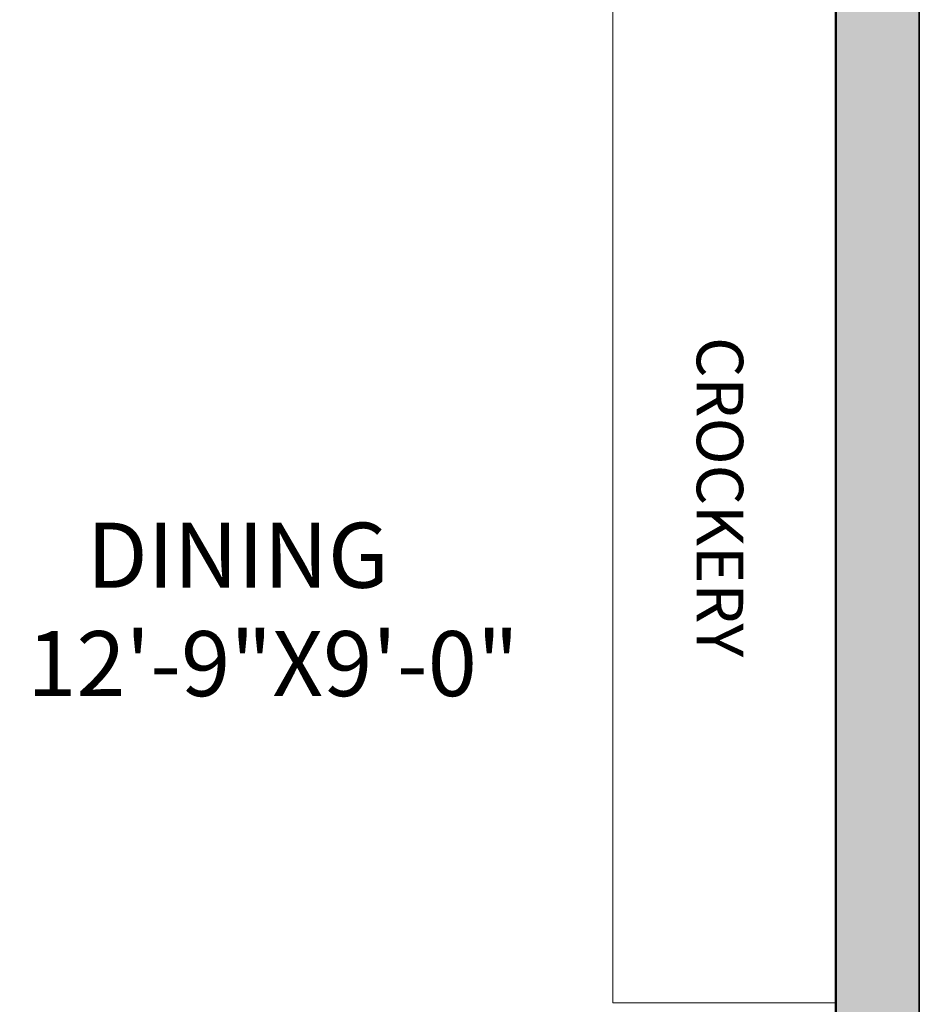
# Model space of a CAD drawing. Units: inches. Extents: x 1734 to 4011, y 1071 to 1891.
# Tile 8 of 27: x 2022 to 2119, y 1650 to 1756. Entities that reach past the tile are written whole.
import ezdxf

# ---------------------------------------------------------------- set-up
doc = ezdxf.new("R2010")
doc.units = ezdxf.units.IN
for name, color, linetype, lineweight in [('A-AREA-IDEN', 3, 'Continuous', 18), ('A-FURN', 8, 'Continuous', 18), ('A-WALL', 7, 'Continuous', 50), ('A-WALL-PATT', 8, 'Continuous', 13), ('C-PROP', 1, 'Continuous', 35)]:
    doc.layers.add(name, color=color, linetype=linetype, lineweight=lineweight)
doc.styles.get("Standard").update_dxf_attribs({"font": 'arial.ttf'})

msp = doc.modelspace()

# ---------------------------------------------------------------- hatches: boundary and pattern name
at = {"layer": 'A-WALL-PATT'}
h = msp.add_hatch(color=256, dxfattribs=at)
h.dxf.hatch_style = 1
h.paths.add_polyline_path([(1857.65, 1835.06), (1857.65, 1793.06), (1862.65, 1793.06), (1862.65, 1835.06), (1951.65, 1835.06), (1951.65, 1763.06), (1897.65, 1763.06), (1897.65, 1758.06), (1951.65, 1758.06), (1951.65, 1617.06), (1956.65, 1617.06), (1956.65, 1758.06), (2009.65, 1758.06), (2009.65, 1763.06), (1956.65, 1763.06), (1956.65, 1835.06), (2044.65, 1835.06), (2044.65, 1763.06), (2039.65, 1763.06), (2039.65, 1758.06), (2054.65, 1758.06), (2054.65, 1763.06), (2049.65, 1763.06), (2049.65, 1835.06), (2109.65, 1835.06), (2109.65, 1763.06), (2084.65, 1763.06), (2084.65, 1758.06), (2109.65, 1758.06), (2109.65, 1530.06), (2095.15, 1530.06), (2095.15, 1525.06), (2109.65, 1525.06), (2109.65, 1471.06), (2089.15, 1471.06), (2089.15, 1466.06), (2109.65, 1466.06), (2109.65, 1250.06), (2015.65, 1250.06), (2015.65, 1241.06), (2109.65, 1241.06), (2109.65, 1133.06), (1952.65, 1133.06), (1952.65, 1197.06), (1953.65, 1197.06), (1953.65, 1202.06), (1946.65, 1202.06), (1946.65, 1133.06), (1934.65, 1133.06), (1934.65, 1124.06), (2118.65, 1124.06), (2118.65, 1844.06), (1758.65, 1844.06), (1758.65, 1758.06), (1773.65, 1758.06), (1773.65, 1763.06), (1767.65, 1763.06), (1767.65, 1835.06)])
h.paths.add_polyline_path([(1803.65, 1649.06), (1812.65, 1649.06), (1812.65, 1758.06), (1867.65, 1758.06), (1867.65, 1763.06), (1797.65, 1763.06), (1797.65, 1758.06), (1803.65, 1758.06)], flags=17)
h.paths.add_polyline_path([(1803.65, 1572.06), (1956.65, 1572.06), (1956.65, 1581.06), (1951.65, 1581.06), (1951.65, 1577.06), (1812.65, 1577.06), (1812.65, 1601.06), (1803.65, 1601.06)], flags=17)
h.paths.add_polyline_path([(2044.65, 1530.06), (2044.65, 1525.06), (2059.15, 1525.06), (2059.15, 1530.06)], flags=17)
h.paths.add_polyline_path([(2009.65, 1466.06), (2035.15, 1466.06), (2035.15, 1471.06), (2014.65, 1471.06), (2014.65, 1530.06), (2009.65, 1530.06)], flags=17)
h.paths.add_polyline_path([(1896.65, 1537.06), (1896.65, 1533.06), (1901.65, 1533.06), (1901.65, 1542.06), (1803.65, 1542.06), (1803.65, 1507.06), (1812.65, 1507.06), (1812.65, 1537.06)], flags=17)
h.paths.add_polyline_path([(1906.65, 1466.06), (1906.65, 1471.06), (1901.65, 1471.06), (1901.65, 1503.06), (1896.65, 1503.06), (1896.65, 1471.06), (1812.65, 1471.06), (1812.65, 1483.06), (1803.65, 1483.06), (1803.65, 1400.06), (1812.65, 1400.06), (1812.65, 1466.06)], flags=17)
h.paths.add_polyline_path([(1951.65, 1334.06), (1909.15, 1334.06), (1909.15, 1325.06), (1956.65, 1325.06), (1956.65, 1466.06), (1961.65, 1466.06), (1961.65, 1471.06), (1942.65, 1471.06), (1942.65, 1466.06), (1951.65, 1466.06)], flags=17)
h.paths.add_polyline_path([(1812.65, 1334.06), (1812.65, 1352.06), (1803.65, 1352.06), (1803.65, 1325.06), (1855.15, 1325.06), (1855.15, 1334.06)], flags=17)
h.paths.add_polyline_path([(1956.65, 1298.06), (1956.65, 1301.06), (1947.65, 1301.06), (1947.65, 1298.06)], flags=17)
h.paths.add_polyline_path([(1967.65, 1241.06), (1967.65, 1250.06), (1947.65, 1250.06), (1947.65, 1241.06)], flags=17)

# ---------------------------------------------------------------- linework, layer by layer
at = {"layer": 'A-FURN'}
for p, q in [((2085.65, 1758.06), (2085.65, 1650.06)), ((2085.65, 1758.06), (2085.65, 1650.06)), ((2085.65, 1650.06), (2109.65, 1650.06))]:
    msp.add_line(p, q, dxfattribs=at)
at = {"layer": 'A-WALL'}
msp.add_line((2109.65, 1758.06), (2109.65, 1530.06), dxfattribs=at)
at = {"layer": 'C-PROP'}
msp.add_lwpolyline([(1814.65, 1124.06), (1758.65, 1124.06), (1758.65, 1844.06), (2118.65, 1844.06), (2118.65, 1124.06), (1934.65, 1124.06)], dxfattribs=at)

# ---------------------------------------------------------------- texts
at = {"layer": 'A-AREA-IDEN', "insert": (2099.68, 1726.32), "char_height": 5, "attachment_point": 1, "rotation": 270}
msp.add_mtext_dynamic_manual_height_columns('   CROCKERY', width=86.9528, gutter_width=12.5, heights=[0], dxfattribs=at)
at = {"layer": 'A-AREA-IDEN', "insert": (2022.57, 1701.74), "char_height": 7, "attachment_point": 1}
msp.add_mtext_dynamic_manual_height_columns('   DINING\\P12\'-9"X9\'-0"', width=86.9528, gutter_width=12.5, heights=[0], dxfattribs=at)

doc.saveas('drawing.dxf')
